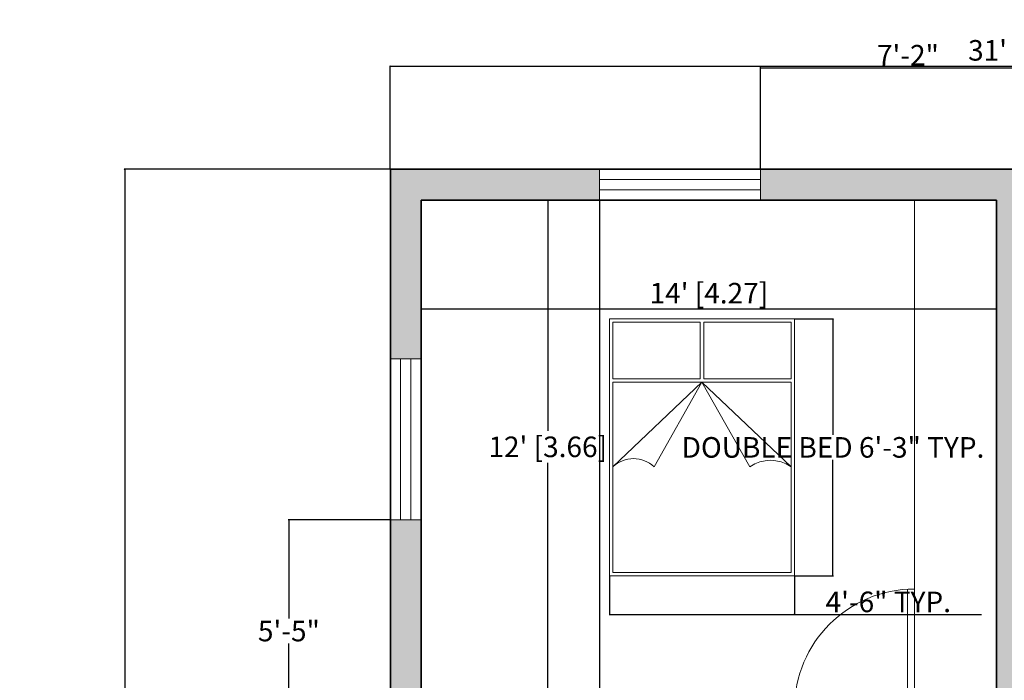
# Model space of a CAD drawing. Units: inches. Extents: x 2322 to 2932, y 142 to 762.
# Tile 5 of 7: x 2322 to 2609, y 570 to 762. Entities that reach past the tile are written whole.
import ezdxf

# ---------------------------------------------------------------- set-up
doc = ezdxf.new("R2010")
doc.units = ezdxf.units.IN
doc.header["$MEASUREMENT"] = 0
for name, color, linetype, lineweight in [('A-ANNO-DIMS', 2, 'Continuous', 18), ('A-DOOR', 3, 'Continuous', 18), ('A-FLOR-CASE', 32, 'Continuous', 18), ('A-GLAZ', 4, 'Continuous', 18), ('A-WALL', 7, 'Continuous', 35)]:
    doc.layers.add(name, color=color, linetype=linetype, lineweight=lineweight)
doc.layers.add('A-WALL-PATT', color=40, linetype='Continuous', lineweight=13, true_color=0xf8d731)
doc.layers.add('Furniture', color=7, linetype='Continuous', lineweight=15, true_color=0xffffff)
doc.styles.get("Standard").update_dxf_attribs({"font": 'italic8.shx'})
doc.dimstyles.get("Standard").update_dxf_attribs({"dimtxt": 6, "dimasz": 0.15, "dimexe": 0.18, "dimexo": 0.0625, "dimgap": 0.09, "dimtad": 1, "dimtih": 1, "dimtoh": 1, "dimzin": 0, "dimdsep": 46, "dimlunit": 3, "dimtxsty": 'Standard', "dimblk": 'CLOSEDBLANK', "dimcen": 0.09, "dimclrd": 3, "dimclre": 1, "dimclrt": 6, "dimadec": 0, "dimazin": 0, "dimtfac": 1, "dimtofl": 0, "dimtmove": 0, "dimatfit": 3, "dimldrblk": 'DOT', "dimfxl": 1, "dimtolj": 1, "dimtzin": 0, "dimarcsym": 0})

# ---------------------------------------------------------------- blocks, each defined once
blk = doc.blocks.new('_ClosedBlank')
at = {"color": 0, "linetype": 'ByBlock', "lineweight": -2}
for p, q in [((-1, 0.2), (0, 0)), ((-1, 0.2), (-1, -0.2)), ((0, 0), (-1, -0.2))]:
    blk.add_line(p, q, dxfattribs=at)
blk = doc.blocks.new('*D7')
at = {"layer": 'A-ANNO-DIMS', "color": 0, "lineweight": -2, "transparency": 16777216}
for p, q in [((2430.06, 718.88), (2430.06, 749.05)), ((2430.21, 748.87), (2801.91, 748.87)), ((2802.06, 718.88), (2802.06, 749.05))]:
    blk.add_line(p, q, dxfattribs=at)
at = {"layer": 'Defpoints', "color": 0, "transparency": 16777216}
for p in [(2802.06, 748.87), (2430.06, 718.82), (2802.06, 718.82)]:
    blk.add_point(p, dxfattribs=at)
at = {"layer": 'A-ANNO-DIMS', "color": 0, "lineweight": -2, "transparency": 16777216, "xscale": 0.15, "yscale": 0.15, "zscale": 0.15, "rotation": 180}
blk.add_blockref('_ClosedBlank', (2430.06, 748.87), dxfattribs=at)
at = {"layer": 'A-ANNO-DIMS', "color": 0, "lineweight": -2, "transparency": 16777216, "xscale": 0.15, "yscale": 0.15, "zscale": 0.15}
blk.add_blockref('_ClosedBlank', (2802.06, 748.87), dxfattribs=at)
at = {"layer": 'A-ANNO-DIMS', "color": 0, "transparency": 16777216, "insert": (2616.06, 753.53), "char_height": 6, "attachment_point": 5}
blk.add_mtext("\\A1;31' [9.45]", dxfattribs=at)
blk = doc.blocks.new('_Dot')
at = {"color": 0, "linetype": 'ByBlock', "lineweight": -2}
blk.add_line((-0.5, 0), (-1, 0), dxfattribs=at)
at = {"color": 0, "linetype": 'ByBlock', "const_width": 0.5}
blk.add_lwpolyline([(-0.25, 0, 1), (0.25, 0, 1)], format="xyb", close=True, dxfattribs=at)
blk = doc.blocks.new('*D8')
at = {"layer": 'A-ANNO-DIMS', "color": 0, "lineweight": -2, "transparency": 16777216}
for p, q in [((2430, 718.82), (2352.33, 718.82)), ((2352.51, 718.67), (2352.51, 501.45)), ((2352.51, 274.91), (2352.51, 492.13)), ((2430, 274.76), (2352.33, 274.76))]:
    blk.add_line(p, q, dxfattribs=at)
at = {"layer": 'Defpoints', "color": 0, "transparency": 16777216}
for p in [(2430.06, 718.82), (2352.51, 274.76), (2430.06, 274.76)]:
    blk.add_point(p, dxfattribs=at)
at = {"layer": 'A-ANNO-DIMS', "color": 0, "lineweight": -2, "transparency": 16777216, "xscale": 0.15, "yscale": 0.15, "zscale": 0.15}
for p, rotation in [((2352.51, 718.82), 90), ((2352.51, 274.76), 270)]:
    blk.add_blockref('_ClosedBlank', p, dxfattribs=dict(at, rotation=rotation))
at = {"layer": 'A-ANNO-DIMS', "color": 0, "transparency": 16777216, "insert": (2352.51, 496.79), "char_height": 6, "attachment_point": 5}
blk.add_mtext('\\A1;37\'-0.06" [11.28]', dxfattribs=at)
blk = doc.blocks.new('*D9')
at = {"layer": 'A-ANNO-DIMS', "color": 0, "lineweight": -2, "transparency": 16777216}
for p, q in [((2460.73, 709.82), (2476.2, 709.82)), ((2476.02, 709.67), (2476.02, 642.48)), ((2476.02, 565.97), (2476.02, 633.16)), ((2460.73, 565.82), (2476.2, 565.82))]:
    blk.add_line(p, q, dxfattribs=at)
at = {"layer": 'Defpoints', "color": 0, "transparency": 16777216}
for p in [(2460.67, 709.82), (2460.67, 565.82), (2476.02, 565.82)]:
    blk.add_point(p, dxfattribs=at)
at = {"layer": 'A-ANNO-DIMS', "color": 0, "lineweight": -2, "transparency": 16777216, "xscale": 0.15, "yscale": 0.15, "zscale": 0.15}
for p, rotation in [((2476.02, 709.82), 90), ((2476.02, 565.82), 270)]:
    blk.add_blockref('_ClosedBlank', p, dxfattribs=dict(at, rotation=rotation))
at = {"layer": 'A-ANNO-DIMS', "color": 0, "transparency": 16777216, "insert": (2476.02, 637.82), "char_height": 6, "attachment_point": 5}
blk.add_mtext("\\A1;12' [3.66]", dxfattribs=at)
blk = doc.blocks.new('*D10')
at = {"layer": 'A-ANNO-DIMS', "color": 0, "lineweight": -2, "transparency": 16777216}
for p, q in [((2439.06, 678.06), (2439.06, 678.18)), ((2606.91, 678), (2439.21, 678)), ((2607.06, 678.06), (2607.06, 678.18))]:
    blk.add_line(p, q, dxfattribs=at)
at = {"layer": 'Defpoints', "color": 0, "transparency": 16777216}
for p in [(2439.06, 678), (2439.06, 678), (2607.06, 678)]:
    blk.add_point(p, dxfattribs=at)
at = {"layer": 'A-ANNO-DIMS', "color": 0, "lineweight": -2, "transparency": 16777216, "xscale": 0.15, "yscale": 0.15, "zscale": 0.15, "rotation": 180}
blk.add_blockref('_ClosedBlank', (2439.06, 678), dxfattribs=at)
at = {"layer": 'A-ANNO-DIMS', "color": 0, "lineweight": -2, "transparency": 16777216, "xscale": 0.15, "yscale": 0.15, "zscale": 0.15}
blk.add_blockref('_ClosedBlank', (2607.06, 678), dxfattribs=at)
at = {"layer": 'A-ANNO-DIMS', "color": 0, "transparency": 16777216, "insert": (2523.06, 682.66), "char_height": 6, "attachment_point": 5}
blk.add_mtext("\\A1;14' [4.27]", dxfattribs=at)
blk = doc.blocks.new('DOOR-SWING-35')
for p, q in [((0, 35), (0, 0)), ((2, 35), (2, 0)), ((0, 0), (35, 0))]:
    blk.add_line(p, q)
blk.add_arc((0, 0), 35, 0, 90)
blk = doc.blocks.new('WINDOW-47X9')
for p, q in [((47, 9), (0, 9)), ((0, 9), (0, 0)), ((47, 0), (47, 9)), ((0, 6), (47, 6)), ((0, 3), (47, 3)), ((0, 0), (47, 0))]:
    blk.add_line(p, q)
blk = doc.blocks.new('BED-DOUBLE')
for p, q in [((0, 75), (54, 75)), ((0, 0), (0, 75)), ((54, 75), (54, 0)), ((1, 74), (26.5, 74)), ((1, 57.55), (1, 74)), ((26.5, 57.55), (26.5, 74)), ((27.5, 74), (53, 74)), ((27.5, 57.55), (27.5, 74)), ((53, 74), (53, 57.55)), ((1, 57.55), (26.5, 57.55)), ((27.5, 57.55), (53, 57.55)), ((1, 1), (1, 56.55)), ((1, 56.55), (53, 56.55)), ((27, 56.55), (1, 31.82)), ((13, 31.82), (27, 56.55)), ((27, 56.55), (53, 31.82)), ((41, 31.82), (27, 56.55)), ((53, 56.55), (53, 1)), ((54, 0), (0, 0)), ((53, 1), (1, 1))]:
    blk.add_line(p, q)
for centre, radius, start, end in [((7, 25.51), 8.71, 46.4371, 133.5629), ((47, 23.41), 10.33, 54.4852, 125.5148)]:
    blk.add_arc(centre, radius, start, end)
blk = doc.blocks.new('*D38')
at = {"layer": 'A-ANNO-DIMS', "color": 1, "lineweight": -2, "transparency": 16777216}
for p, q in [((2548.12, 675.16), (2559.48, 675.16)), ((2548.12, 600.16), (2559.48, 600.16))]:
    blk.add_line(p, q, dxfattribs=at)
at = {"layer": 'A-ANNO-DIMS', "color": 3, "lineweight": -2, "transparency": 16777216}
for p, q in [((2559.3, 675.01), (2559.3, 641.32)), ((2559.3, 600.31), (2559.3, 634))]:
    blk.add_line(p, q, dxfattribs=at)
at = {"layer": 'Defpoints', "color": 0, "transparency": 16777216}
for p in [(2548.05, 675.16), (2559.3, 675.16), (2548.05, 600.16)]:
    blk.add_point(p, dxfattribs=at)
at = {"layer": 'A-ANNO-DIMS', "color": 3, "lineweight": -2, "transparency": 16777216, "xscale": 0.15, "yscale": 0.15, "zscale": 0.15}
for p, rotation in [((2559.3, 675.16), 90), ((2559.3, 600.16), 270)]:
    blk.add_blockref('_ClosedBlank', p, dxfattribs=dict(at, rotation=rotation))
at = {"layer": 'A-ANNO-DIMS', "color": 6, "transparency": 16777216, "insert": (2559.3, 637.66), "char_height": 6, "attachment_point": 5}
blk.add_mtext('\\A1;DOUBLE BED 6\'-3" TYP.', dxfattribs=at)
blk = doc.blocks.new('*D39')
at = {"layer": 'A-ANNO-DIMS', "color": 1, "lineweight": -2, "transparency": 16777216}
for p, q in [((2494.05, 600.1), (2494.05, 588.73)), ((2548.05, 600.1), (2548.05, 588.73))]:
    blk.add_line(p, q, dxfattribs=at)
at = {"layer": 'A-ANNO-DIMS', "color": 3, "lineweight": -2, "transparency": 16777216}
for p, q in [((2494.2, 588.91), (2547.9, 588.91)), ((2548.05, 588.91), (2602.67, 588.91))]:
    blk.add_line(p, q, dxfattribs=at)
at = {"layer": 'Defpoints', "color": 0, "transparency": 16777216}
for p in [(2494.05, 600.16), (2548.05, 600.16), (2548.05, 588.91)]:
    blk.add_point(p, dxfattribs=at)
at = {"layer": 'A-ANNO-DIMS', "color": 3, "lineweight": -2, "transparency": 16777216, "xscale": 0.15, "yscale": 0.15, "zscale": 0.15, "rotation": 180}
blk.add_blockref('_ClosedBlank', (2494.05, 588.91), dxfattribs=at)
at = {"layer": 'A-ANNO-DIMS', "color": 3, "lineweight": -2, "transparency": 16777216, "xscale": 0.15, "yscale": 0.15, "zscale": 0.15}
blk.add_blockref('_ClosedBlank', (2548.05, 588.91), dxfattribs=at)
at = {"layer": 'A-ANNO-DIMS', "color": 6, "transparency": 16777216, "insert": (2575.44, 592.57), "char_height": 6, "attachment_point": 5}
blk.add_mtext('\\A1;4\'-6" TYP.', dxfattribs=at)
blk = doc.blocks.new('*D51')
at = {"layer": 'A-ANNO-DIMS', "color": 1, "lineweight": -2, "transparency": 16777216}
for p, q in [((2439.06, 709.76), (2439.06, 146.01)), ((2491.1, 709.76), (2491.1, 146.01))]:
    blk.add_line(p, q, dxfattribs=at)
at = {"layer": 'A-ANNO-DIMS', "color": 3, "lineweight": -2, "transparency": 16777216}
blk.add_line((2439.21, 146.19), (2490.95, 146.19), dxfattribs=at)
at = {"layer": 'Defpoints', "color": 0, "transparency": 16777216}
for p in [(2439.06, 709.82), (2491.1, 709.82), (2491.1, 146.19)]:
    blk.add_point(p, dxfattribs=at)
at = {"layer": 'A-ANNO-DIMS', "color": 3, "lineweight": -2, "transparency": 16777216, "xscale": 0.15, "yscale": 0.15, "zscale": 0.15, "rotation": 180}
blk.add_blockref('_ClosedBlank', (2439.06, 146.19), dxfattribs=at)
at = {"layer": 'A-ANNO-DIMS', "color": 3, "lineweight": -2, "transparency": 16777216, "xscale": 0.15, "yscale": 0.15, "zscale": 0.15}
blk.add_blockref('_ClosedBlank', (2491.1, 146.19), dxfattribs=at)
at = {"layer": 'A-ANNO-DIMS', "color": 6, "transparency": 16777216, "insert": (2465.08, 149.85), "char_height": 6, "attachment_point": 5}
blk.add_mtext('\\A1;4\'-4"', dxfattribs=at)
blk = doc.blocks.new('*D52')
at = {"layer": 'A-ANNO-DIMS', "color": 1, "lineweight": -2, "transparency": 16777216}
for p, q in [((2538.1, 718.88), (2538.1, 748.62)), ((2624.25, 718.88), (2624.25, 748.62))]:
    blk.add_line(p, q, dxfattribs=at)
at = {"layer": 'A-ANNO-DIMS', "color": 3, "lineweight": -2, "transparency": 16777216}
blk.add_line((2538.25, 748.44), (2624.1, 748.44), dxfattribs=at)
at = {"layer": 'Defpoints', "color": 0, "transparency": 16777216}
for p in [(2624.25, 748.44), (2538.1, 718.82), (2624.25, 718.82)]:
    blk.add_point(p, dxfattribs=at)
at = {"layer": 'A-ANNO-DIMS', "color": 3, "lineweight": -2, "transparency": 16777216, "xscale": 0.15, "yscale": 0.15, "zscale": 0.15, "rotation": 180}
blk.add_blockref('_ClosedBlank', (2538.1, 748.44), dxfattribs=at)
at = {"layer": 'A-ANNO-DIMS', "color": 3, "lineweight": -2, "transparency": 16777216, "xscale": 0.15, "yscale": 0.15, "zscale": 0.15}
blk.add_blockref('_ClosedBlank', (2624.25, 748.44), dxfattribs=at)
at = {"layer": 'A-ANNO-DIMS', "color": 6, "transparency": 16777216, "insert": (2581.17, 752.1), "char_height": 6, "attachment_point": 5}
blk.add_mtext('\\A1;7\'-2"', dxfattribs=at)
blk = doc.blocks.new('*D60')
at = {"layer": 'A-ANNO-DIMS', "color": 1, "lineweight": -2, "transparency": 16777216}
for p, q in [((2430, 616.55), (2400.26, 616.55)), ((2430, 551.56), (2400.26, 551.56))]:
    blk.add_line(p, q, dxfattribs=at)
at = {"layer": 'A-ANNO-DIMS', "color": 3, "lineweight": -2, "transparency": 16777216}
for p, q in [((2400.44, 616.4), (2400.44, 587.72)), ((2400.44, 551.71), (2400.44, 580.39))]:
    blk.add_line(p, q, dxfattribs=at)
at = {"layer": 'Defpoints', "color": 0, "transparency": 16777216}
for p in [(2400.44, 616.55), (2430.06, 616.55), (2430.06, 551.56)]:
    blk.add_point(p, dxfattribs=at)
at = {"layer": 'A-ANNO-DIMS', "color": 3, "lineweight": -2, "transparency": 16777216, "xscale": 0.15, "yscale": 0.15, "zscale": 0.15}
for p, rotation in [((2400.44, 616.55), 90), ((2400.44, 551.56), 270)]:
    blk.add_blockref('_ClosedBlank', p, dxfattribs=dict(at, rotation=rotation))
at = {"layer": 'A-ANNO-DIMS', "color": 6, "transparency": 16777216, "insert": (2400.44, 584.06), "char_height": 6, "attachment_point": 5}
blk.add_mtext('\\A1;5\'-5"', dxfattribs=at)

msp = doc.modelspace()

# ---------------------------------------------------------------- hatches: boundary and pattern name
at = {"layer": 'A-WALL-PATT'}
h = msp.add_hatch(color=256, dxfattribs=at)
h.dxf.hatch_style = 1
h.paths.add_polyline_path([(2439.065, 709.819), (2491.097, 709.819), (2491.097, 718.819), (2430.065, 718.819), (2430.065, 663.548), (2439.065, 663.548)])
h.paths.add_polyline_path([(2704.233, 718.819), (2654.246, 718.819), (2654.246, 709.819), (2668.565, 709.819), (2668.565, 661.819), (2673.065, 661.819), (2673.065, 709.819), (2704.233, 709.819)], flags=17)
h.paths.add_polyline_path([(2624.246, 718.819), (2538.097, 718.819), (2538.097, 709.819), (2607.065, 709.819), (2607.065, 565.819), (2583.065, 565.819), (2583.065, 561.319), (2611.565, 561.319), (2611.565, 609.319), (2668.565, 609.319), (2668.565, 561.319), (2758.065, 561.319), (2758.065, 565.819), (2673.065, 565.819), (2673.065, 626.819), (2668.565, 626.819), (2668.565, 613.819), (2611.565, 613.819), (2611.565, 709.819), (2624.246, 709.819)])
h.paths.add_polyline_path([(2802.065, 718.819), (2751.233, 718.819), (2751.233, 709.819), (2793.065, 709.819), (2793.065, 660.138), (2802.065, 660.138)])
h.paths.add_polyline_path([(2802.065, 613.138), (2793.065, 613.138), (2793.065, 478.568), (2802.065, 478.568)])
h.paths.add_polyline_path([(2439.065, 616.548), (2430.065, 616.548), (2430.065, 551.562), (2439.065, 551.562), (2439.065, 561.319), (2483.455, 561.319), (2483.455, 565.819), (2439.065, 565.819)])
h.paths.add_polyline_path([(2548.065, 565.819), (2518.455, 565.819), (2518.455, 561.319), (2541.065, 561.319), (2541.065, 501.319), (2439.065, 501.319), (2439.065, 516.562), (2430.065, 516.562), (2430.065, 465.181), (2439.065, 465.181), (2439.065, 496.819), (2503.266, 496.819), (2541.065, 496.819), (2541.065, 472.819), (2545.565, 472.819), (2545.565, 561.319), (2548.065, 561.319)])
h.paths.add_polyline_path([(2439.065, 418.181), (2430.065, 418.181), (2430.065, 342.453), (2439.065, 342.453), (2439.065, 367.819), (2602.565, 367.819), (2602.565, 283.756), (2594.693, 283.756), (2594.693, 274.756), (2611.565, 274.756), (2611.565, 501.319), (2580.942, 501.319), (2580.942, 496.819), (2607.065, 496.819), (2607.065, 376.819), (2439.065, 376.819)])
h.paths.add_polyline_path([(2793.057, 530.805), (2793.057, 530.68), (2793.106, 530.68), (2793.106, 530.805)], flags=25)
h.paths.add_polyline_path([(2793.057, 530.808), (2793.057, 530.676), (2793.106, 530.676), (2793.106, 530.808)], flags=9)

# ---------------------------------------------------------------- linework, layer by layer
at = {"layer": 'A-FLOR-CASE'}
msp.add_line((2583.065, 561.319), (2583.065, 709.819), dxfattribs=at)
at = {"layer": 'A-WALL'}
for p, q in [((2802.065, 718.819), (2430.065, 718.819)), ((2430.065, 718.819), (2430.065, 274.756)), ((2439.065, 709.819), (2439.065, 565.819)), ((2607.065, 709.819), (2439.065, 709.819)), ((2607.065, 709.819), (2607.065, 565.819))]:
    msp.add_line(p, q, dxfattribs=at)

# ---------------------------------------------------------------- block references
at = {"layer": 'A-DOOR', "extrusion": (0, 0, -1), "zscale": -1}
msp.add_blockref('DOOR-SWING-35', (-2583.064, 561.319), dxfattribs=at)
at = {"layer": 'A-GLAZ'}
msp.add_blockref('WINDOW-47X9', (2491.097, 709.819), dxfattribs=at)
at = {"layer": 'A-GLAZ', "rotation": 90.00000000000188}
msp.add_blockref('WINDOW-47X9', (2439.064, 616.548), dxfattribs=at)
at = {"layer": 'Furniture'}
msp.add_blockref('BED-DOUBLE', (2494.053, 600.157), dxfattribs=at)

# ---------------------------------------------------------------- dimensions: what is measured, and where the dimension line sits
at = {"layer": 'A-ANNO-DIMS'}
for base, p1, p2, override, picture, middle in [((2802.065, 748.867), (2430.065, 718.819), (2802.065, 718.819), {"dimclrd": 0, "dimclre": 0, "dimclrt": 0}, '*D7', (2616.065, 753.528)), ((2624.246, 748.444), (2538.097, 718.819), (2624.246, 718.819), {"dimdec": 1, "dimlfac": 1, "dimrnd": 0, "dimzin": 1, "dimdsep": 46, "dimlunit": 4, "dimfrac": 2}, '*D52', (2581.172, 752.105)), ((2491.097, 146.194), (2439.065, 709.819), (2491.097, 709.819), {"dimdec": 1, "dimlfac": 1, "dimrnd": 0, "dimzin": 1, "dimdsep": 46, "dimlunit": 4, "dimfrac": 2}, '*D51', (2465.081, 149.855)), ((2439.065, 678.001), (2607.065, 678.001), (2439.065, 678.001), {"dimclrd": 0, "dimclre": 0, "dimclrt": 0}, '*D10', (2523.065, 682.662))]:
    dim = msp.add_linear_dim(base=base, p1=p1, p2=p2, dimstyle='Standard', override=override, dxfattribs=at)
    dim.commit()
    dim.dimension.update_dxf_attribs({"geometry": picture, "text_midpoint": middle})
for base, p1, p2, override, picture, middle in [((2352.512, 274.756), (2430.065, 718.819), (2430.065, 274.756), {"dimclrd": 0, "dimclre": 0, "dimclrt": 0}, '*D8', (2352.512, 496.787)), ((2476.019, 565.819), (2460.669, 709.819), (2460.669, 565.819), {"dimclrd": 0, "dimclre": 0, "dimclrt": 0}, '*D9', (2476.019, 637.819)), ((2400.44, 616.548), (2430.065, 551.562), (2430.065, 616.548), {"dimdec": 1, "dimlfac": 1, "dimrnd": 0, "dimzin": 1, "dimdsep": 46, "dimlunit": 4, "dimfrac": 2}, '*D60', (2400.44, 584.055))]:
    dim = msp.add_linear_dim(base=base, p1=p1, p2=p2, angle=90, dimstyle='Standard', override=override, dxfattribs=at)
    dim.commit()
    dim.dimension.update_dxf_attribs({"geometry": picture, "text_midpoint": middle})
dim = msp.add_linear_dim(base=(2559.303, 675.158), p1=(2548.053, 600.158), p2=(2548.053, 675.158), angle=90, text='DOUBLE BED <> TYP.', dimstyle='Standard', override={"dimdec": 1, "dimlfac": 1, "dimrnd": 0, "dimzin": 1, "dimdsep": 46, "dimlunit": 4, "dimfrac": 2}, dxfattribs=at)
dim.commit()
dim.dimension.update_dxf_attribs({"geometry": '*D38', "text_midpoint": (2559.303, 637.658)})
dim = msp.add_linear_dim(base=(2548.053, 588.908), p1=(2494.053, 600.158), p2=(2548.053, 600.158), text='<> TYP.', dimstyle='Standard', override={"dimdec": 1, "dimlfac": 1, "dimrnd": 0, "dimzin": 1, "dimdsep": 46, "dimlunit": 4, "dimfrac": 2}, dxfattribs=at)
dim.commit()
dim.dimension.update_dxf_attribs({"geometry": '*D39', "text_midpoint": (2575.436, 592.569)})

doc.saveas('drawing.dxf')
